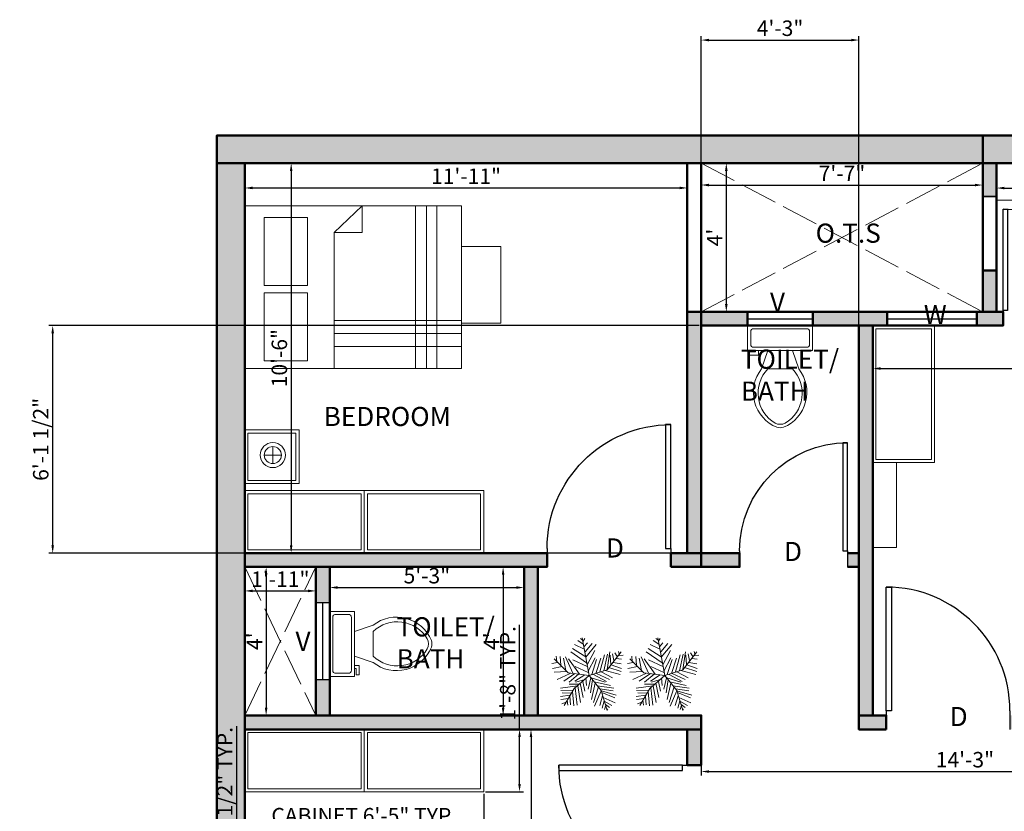
# Model space of a CAD drawing. Units: inches. Extents: x 2227 to 2709, y 1385 to 2029.
# Tile 3 of 4: x 2227 to 2545, y 1773 to 2029. Entities that reach past the tile are written whole.
import ezdxf

# ---------------------------------------------------------------- set-up
doc = ezdxf.new("R2010")
doc.units = ezdxf.units.IN
doc.linetypes.add('ACAD_ISO02W100', pattern=[15, 12, -3])
for name, color, linetype, lineweight in [('A-ANNO-DIMS', 1, 'Continuous', 18), ('A-ANNO-TEXT', 30, 'Continuous', 18), ('A-AREA-IDEN', 30, 'Continuous', 25), ('A-FLOR-FIXT', 9, 'Continuous', 18), ('A-FLOR-OPEN', 8, 'ACAD_ISO02W100', 18), ('A-FURN', 50, 'Continuous', 18), ('A-WALL-HIDN', 160, 'ACAD_ISO02W100', 18), ('A-WALL-PATT', 252, 'Continuous', 13), ('BED', 50, 'Continuous', 18), ('DOOR', 130, 'Continuous', 25), ('TREE', 80, 'Continuous', 13), ('WALL', 160, 'Continuous', 50), ('WIND', 40, 'Continuous', 25)]:
    doc.layers.add(name, color=color, linetype=linetype, lineweight=lineweight)
doc.styles.get("Standard").update_dxf_attribs({"font": 'arial.ttf'})
doc.dimstyles.new('ISO-25', dxfattribs={"dimtxt": 5, "dimasz": 2.5, "dimexe": 1.25, "dimexo": 0.625, "dimtad": 1, "dimdec": 0, "dimlunit": 4, "dimtxsty": 'Standard', "dimcen": 2.5, "dimadec": 0, "dimazin": 0, "dimtfac": 1, "dimtdec": 0, "dimtmove": 0, "dimatfit": 3, "dimfxl": 1, "dimarcsym": 0})

# ---------------------------------------------------------------- blocks, each defined once
blk = doc.blocks.new('*U2')
for p, q in [((0, 0), (0, -6)), ((40, 0), (40, -6))]:
    blk.add_line(p, q)
blk.add_lwpolyline([(0, 0), (0, 40), (1.75, 40), (1.75, 0)], close=True)
blk.add_arc((0, 0), 40, 0, 90)
blk = doc.blocks.new('*U4')
for p, q in [((9.5, -6), (9.5, -2)), ((-10, -8.5), (-8, -8.5)), ((-10, -9.5), (-10, -8.5)), ((-7, -9.5), (-10, -9.5)), ((-8, -8.5), (-8, -8)), ((-7, -8), (-7, -9.5)), ((-4, -8), (-6, -14)), ((4, -8), (6, -14)), ((4, -14), (-4, -14))]:
    blk.add_line(p, q)
blk.add_lwpolyline([(10.5, -8), (10.5, 0), (-10.5, 0), (-10.5, -8)], close=True)
for points in [[(-9.5, -2), (-9.5, -6)], [(8.5, -1), (-8.5, -1)], [(-8.5, -7), (8.5, -7)]]:
    blk.add_lwpolyline(points)
for centre, radius, start, end in [((-8.62, -1.88), 0.884, 81.8699, 188.1301), ((8.62, -1.88), 0.884, 351.8699, 98.1301), ((-8.62, -6.12), 0.884, 171.8699, 278.1301), ((8.62, -6.12), 0.884, 261.8699, 8.1301), ((3.52, -21.58), 12.17, 141.4691, 247.9714), ((4.2, -21.82), 11.33, 136.3677, 238.9468), ((-3.52, -21.58), 12.17, 292.0284, 38.5307), ((-4.2, -21.82), 11.33, 301.053, 43.6321), ((0, -27.88), 4, 245.7318, 294.2682), ((0, -29), 4, 254.8605, 285.1395)]:
    blk.add_arc(centre, radius, start, end)
blk = doc.blocks.new('*U6')
for p, q in [((-7.288, 39.707), (-21.778, 46.673)), ((-8.737, 47.138), (-17.069, 52.711)), ((-10.186, 53.64), (-13.084, 55.962)), ((0, 0), (-10.5, 57)), ((-9.099, 51.782), (-6.563, 55.962)), ((-7.65, 43.423), (-2.578, 49.46)), ((-5.839, 35.992), (4.667, 48.067)), ((-5.114, 27.632), (10.463, 46.673)), ((-3.665, 19.273), (-27.574, 35.527)), ((-5.114, 28.097), (-24.676, 40.636)), ((-2.941, 16.486), (8.652, 37.85)), ((16.259, 5.805), (23.142, 31.348)), ((22.055, 7.198), (27.489, 32.277)), ((27, 9), (48, 36)), ((27.127, 9.056), (31.112, 35.992)), ((31.836, 30.883), (32.561, 16.486)), ((35.096, 32.741), (37.27, 22.524)), ((38.719, 34.134), (41.979, 28.561)), ((43.791, 29.954), (51.036, 30.883)), ((44.153, 36.456), (45.239, 32.741)), ((-47.498, 19.737), (-55.83, 18.344)), ((-31.5, 4.5), (-52.5, 25.5)), ((-48.585, 21.131), (-49.309, 29.026)), ((-43.513, 28.561), (-42.427, 15.558)), ((-38.442, 26.239), (-34.819, 7.663)), ((-35.544, 28.097), (-24.314, 3.947)), ((-14.533, 2.09), (-30.834, 25.31)), ((-24.314, 23.917), (-2.941, 13.7)), ((-1.129, 6.734), (9.014, 26.704)), ((3.942, 1.625), (11.187, 24.381)), ((10.101, 3.483), (17.708, 26.239)), ((33.285, 16.486), (48.862, 10.913)), ((36.183, 19.737), (48.137, 17.88)), ((40.53, 25.775), (48.862, 24.846)), ((-40.615, 13.7), (-55.105, 10.913)), ((-33.37, 6.269), (-52.207, 5.34)), ((-28.299, 3.483), (-47.86, -5.805)), ((-21.416, 3.018), (-38.079, -8.128)), ((0, 0), (-31.5, 4.5)), ((-15.982, 2.09), (-30.11, -9.521)), ((0, 0), (-22.5, -19.5)), ((-6.563, 1.161), (-21.416, -8.128)), ((-20.691, 13.7), (-1.129, 4.876)), ((0, 0), (27, 9)), ((0, 0), (18, -22.5)), ((6.478, 1.625), (26.04, -8.592)), ((11.187, 3.483), (30.749, -5.805)), ((18.07, 5.805), (35.096, -3.483)), ((24.229, 7.663), (46.688, 1.625)), ((29.662, 12.307), (48.137, 6.269)), ((-15.257, -12.772), (-30.11, -12.772)), ((-6.563, -5.805), (-19.967, -9.985)), ((-13.446, -11.378), (-8.737, -32.741)), ((-9.461, -8.592), (-6.201, -23.453)), ((-4.752, -3.483), (-3.665, -14.629)), ((2.493, -3.019), (-1.491, -20.202)), ((1.769, -2.555), (24.229, -9.521)), ((5.029, -6.27), (2.131, -25.775)), ((9.014, -11.378), (3.58, -35.992)), ((7.565, -9.056), (32.198, -14.629)), ((-17.431, -15.094), (-42.789, -18.809)), ((-28.299, -29.026), (-42.789, -31.348)), ((-24.314, -21.596), (-42.427, -22.06)), ((-26.849, -26.24), (-40.253, -25.775)), ((-22.5, -19.5), (-37.5, -45)), ((-25.038, -23.918), (-22.865, -45.281)), ((-20.691, -18.345), (-17.793, -44.352)), ((-17.069, -15.094), (-12.721, -40.172)), ((14.085, -16.951), (6.478, -40.172)), ((18.07, -22.524), (8.289, -45.745)), ((12.274, -15.094), (36.907, -18.809)), ((16.259, -19.738), (36.183, -22.989)), ((18, -22.5), (27, -52.5)), ((18.433, -22.524), (40.53, -29.026)), ((19.157, -25.311), (38.719, -33.206)), ((-30.834, -34.135), (-42.427, -35.528)), ((-34.457, -39.708), (-40.978, -42.494)), ((-32.646, -36.921), (-31.921, -44.352)), ((-29.023, -30.884), (-27.936, -43.887)), ((20.244, -30.419), (15.897, -44.816)), ((22.78, -37.85), (19.519, -48.532)), ((21.331, -32.741), (39.081, -40.636)), ((22.78, -38.314), (34.372, -44.816)), ((24.591, -43.423), (30.749, -47.603)), ((24.591, -45.745), (23.142, -50.854)), ((26.764, -49.925), (28.213, -50.854))]:
    blk.add_line(p, q)
blk = doc.blocks.new('*D9')
at = {"layer": 'A-ANNO-DIMS', "color": 0, "lineweight": -2, "transparency": 16777216}
for p, q in [((2299.71, 1981.71), (2299.71, 1973.09)), ((2442.71, 1981.71), (2442.71, 1973.09)), ((2302.21, 1974.34), (2440.21, 1974.34))]:
    blk.add_line(p, q, dxfattribs=at)
at = {"layer": 'A-ANNO-DIMS', "color": 0, "lineweight": 100, "transparency": 16777216}
for points in [[(2302.21, 1974.76), (2302.21, 1973.93), (2299.71, 1974.34)], [(2440.21, 1974.76), (2440.21, 1973.93), (2442.71, 1974.34)]]:
    blk.add_solid(points, dxfattribs=at)
at = {"layer": 'Defpoints', "color": 0, "lineweight": 100, "transparency": 16777216}
for p in [(2299.71, 1982.33), (2442.71, 1982.33), (2442.71, 1974.34)]:
    blk.add_point(p, dxfattribs=at)
at = {"layer": 'A-ANNO-DIMS', "color": 0, "transparency": 16777216, "insert": (2371.21, 1977.48), "char_height": 5, "attachment_point": 5}
blk.add_mtext('11\'-11"', dxfattribs=at)
blk = doc.blocks.new('*D10')
at = {"layer": 'A-ANNO-DIMS', "color": 0, "lineweight": -2, "transparency": 16777216}
for p, q in [((2300.34, 1982.33), (2315.95, 1982.33)), ((2314.7, 1979.83), (2314.7, 1858.83)), ((2300.34, 1856.33), (2315.95, 1856.33))]:
    blk.add_line(p, q, dxfattribs=at)
at = {"layer": 'A-ANNO-DIMS', "color": 0, "lineweight": 100, "transparency": 16777216}
for points in [[(2314.28, 1979.83), (2315.11, 1979.83), (2314.7, 1982.33)], [(2314.28, 1858.83), (2315.11, 1858.83), (2314.7, 1856.33)]]:
    blk.add_solid(points, dxfattribs=at)
at = {"layer": 'Defpoints', "color": 0, "lineweight": 100, "transparency": 16777216}
for p in [(2299.71, 1982.33), (2299.71, 1856.33), (2314.7, 1856.33)]:
    blk.add_point(p, dxfattribs=at)
at = {"layer": 'A-ANNO-DIMS', "color": 0, "transparency": 16777216, "insert": (2311.52, 1919.33), "char_height": 5, "attachment_point": 5, "rotation": 90}
blk.add_mtext('10\'-6"', dxfattribs=at)
blk = doc.blocks.new('*D11')
at = {"layer": 'A-ANNO-DIMS', "color": 0, "lineweight": -2, "transparency": 16777216}
for p, q in [((2447.21, 1981.71), (2447.21, 1974.03)), ((2538.21, 1981.71), (2538.21, 1974.03)), ((2449.71, 1975.28), (2535.71, 1975.28))]:
    blk.add_line(p, q, dxfattribs=at)
at = {"layer": 'A-ANNO-DIMS', "color": 0, "lineweight": 100, "transparency": 16777216}
for points in [[(2449.71, 1975.7), (2449.71, 1974.86), (2447.21, 1975.28)], [(2535.71, 1975.7), (2535.71, 1974.86), (2538.21, 1975.28)]]:
    blk.add_solid(points, dxfattribs=at)
at = {"layer": 'Defpoints', "color": 0, "lineweight": 100, "transparency": 16777216}
for p in [(2447.21, 1982.33), (2538.21, 1982.33), (2538.21, 1975.28)]:
    blk.add_point(p, dxfattribs=at)
at = {"layer": 'A-ANNO-DIMS', "color": 0, "transparency": 16777216, "insert": (2492.71, 1978.4), "char_height": 5, "attachment_point": 5}
blk.add_mtext('7\'-7"', dxfattribs=at)
blk = doc.blocks.new('*D12')
at = {"layer": 'A-ANNO-DIMS', "color": 0, "lineweight": -2, "transparency": 16777216}
for p, q in [((2447.84, 1982.33), (2456.58, 1982.33)), ((2455.33, 1979.83), (2455.33, 1936.83)), ((2447.84, 1934.33), (2456.58, 1934.33))]:
    blk.add_line(p, q, dxfattribs=at)
at = {"layer": 'A-ANNO-DIMS', "color": 0, "lineweight": 100, "transparency": 16777216}
for points in [[(2454.91, 1979.83), (2455.75, 1979.83), (2455.33, 1982.33)], [(2454.91, 1936.83), (2455.75, 1936.83), (2455.33, 1934.33)]]:
    blk.add_solid(points, dxfattribs=at)
at = {"layer": 'Defpoints', "color": 0, "lineweight": 100, "transparency": 16777216}
for p in [(2447.21, 1982.33), (2447.21, 1934.33), (2455.33, 1934.33)]:
    blk.add_point(p, dxfattribs=at)
at = {"layer": 'A-ANNO-DIMS', "color": 0, "transparency": 16777216, "insert": (2452.21, 1958.33), "char_height": 5, "attachment_point": 5, "rotation": 90}
blk.add_mtext("4'", dxfattribs=at)
blk = doc.blocks.new('*D13')
at = {"layer": 'A-ANNO-DIMS', "color": 0, "lineweight": -2, "transparency": 16777216}
for p, q in [((2542.71, 1981.71), (2542.71, 1973.06)), ((2617.71, 1981.71), (2617.71, 1973.06)), ((2545.21, 1974.31), (2615.21, 1974.31))]:
    blk.add_line(p, q, dxfattribs=at)
at = {"layer": 'A-ANNO-DIMS', "color": 0, "lineweight": 100, "transparency": 16777216}
for points in [[(2545.21, 1974.72), (2545.21, 1973.89), (2542.71, 1974.31)], [(2615.21, 1974.72), (2615.21, 1973.89), (2617.71, 1974.31)]]:
    blk.add_solid(points, dxfattribs=at)
at = {"layer": 'Defpoints', "color": 0, "lineweight": 100, "transparency": 16777216}
for p in [(2542.71, 1982.33), (2617.71, 1982.33), (2617.71, 1974.31)]:
    blk.add_point(p, dxfattribs=at)
at = {"layer": 'A-ANNO-DIMS', "color": 0, "transparency": 16777216, "insert": (2580.21, 1977.49), "char_height": 5, "attachment_point": 5}
blk.add_mtext('6\'-3"', dxfattribs=at)
blk = doc.blocks.new('*D16')
at = {"layer": 'A-ANNO-DIMS', "color": 0, "lineweight": -2, "transparency": 16777216}
for p, q in [((2502.71, 1804.46), (2502.71, 1917.22)), ((2505.21, 1915.97), (2615.21, 1915.97)), ((2617.71, 1804.46), (2617.71, 1917.22))]:
    blk.add_line(p, q, dxfattribs=at)
at = {"layer": 'A-ANNO-DIMS', "color": 0, "lineweight": 100, "transparency": 16777216}
for points in [[(2505.21, 1916.39), (2505.21, 1915.56), (2502.71, 1915.97)], [(2615.21, 1916.39), (2615.21, 1915.56), (2617.71, 1915.97)]]:
    blk.add_solid(points, dxfattribs=at)
at = {"layer": 'Defpoints', "color": 0, "lineweight": 100, "transparency": 16777216}
for p in [(2617.71, 1915.97), (2502.71, 1803.83), (2617.71, 1803.83)]:
    blk.add_point(p, dxfattribs=at)
at = {"layer": 'A-ANNO-DIMS', "color": 0, "transparency": 16777216, "insert": (2560.21, 1919.15), "char_height": 5, "attachment_point": 5}
blk.add_mtext('9\'-7"', dxfattribs=at)
blk = doc.blocks.new('*D17')
at = {"layer": 'A-ANNO-DIMS', "color": 0, "lineweight": -2, "transparency": 16777216}
for p, q in [((2299.71, 1851.21), (2299.71, 1842.84)), ((2322.67, 1851.21), (2322.67, 1842.84)), ((2302.21, 1844.09), (2320.17, 1844.09))]:
    blk.add_line(p, q, dxfattribs=at)
at = {"layer": 'A-ANNO-DIMS', "color": 0, "lineweight": 100, "transparency": 16777216}
for points in [[(2302.21, 1844.51), (2302.21, 1843.68), (2299.71, 1844.09)], [(2320.17, 1844.51), (2320.17, 1843.68), (2322.67, 1844.09)]]:
    blk.add_solid(points, dxfattribs=at)
at = {"layer": 'Defpoints', "color": 0, "lineweight": 100, "transparency": 16777216}
for p in [(2299.71, 1851.83), (2322.67, 1851.83), (2322.67, 1844.09)]:
    blk.add_point(p, dxfattribs=at)
at = {"layer": 'A-ANNO-DIMS', "color": 0, "transparency": 16777216, "insert": (2311.19, 1847.23), "char_height": 5, "attachment_point": 5}
blk.add_mtext('1\'-11"', dxfattribs=at)
blk = doc.blocks.new('*D18')
at = {"layer": 'A-ANNO-DIMS', "color": 0, "lineweight": -2, "transparency": 16777216}
for p, q in [((2300.34, 1851.83), (2307.86, 1851.83)), ((2306.61, 1849.33), (2306.61, 1806.33)), ((2300.34, 1803.83), (2307.86, 1803.83))]:
    blk.add_line(p, q, dxfattribs=at)
at = {"layer": 'A-ANNO-DIMS', "color": 0, "lineweight": 100, "transparency": 16777216}
for points in [[(2306.19, 1849.33), (2307.02, 1849.33), (2306.61, 1851.83)], [(2306.19, 1806.33), (2307.02, 1806.33), (2306.61, 1803.83)]]:
    blk.add_solid(points, dxfattribs=at)
at = {"layer": 'Defpoints', "color": 0, "lineweight": 100, "transparency": 16777216}
for p in [(2299.71, 1851.83), (2299.71, 1803.83), (2306.61, 1803.83)]:
    blk.add_point(p, dxfattribs=at)
at = {"layer": 'A-ANNO-DIMS', "color": 0, "transparency": 16777216, "insert": (2303.48, 1827.83), "char_height": 5, "attachment_point": 5, "rotation": 90}
blk.add_mtext("4'", dxfattribs=at)
blk = doc.blocks.new('*D19')
at = {"layer": 'A-ANNO-DIMS', "color": 0, "lineweight": -2, "transparency": 16777216}
for p, q in [((2327.17, 1851.21), (2327.17, 1843.93)), ((2389.95, 1851.21), (2389.95, 1843.93)), ((2329.67, 1845.18), (2387.45, 1845.18))]:
    blk.add_line(p, q, dxfattribs=at)
at = {"layer": 'A-ANNO-DIMS', "color": 0, "lineweight": 100, "transparency": 16777216}
for points in [[(2329.67, 1845.6), (2329.67, 1844.77), (2327.17, 1845.18)], [(2387.45, 1845.6), (2387.45, 1844.77), (2389.95, 1845.18)]]:
    blk.add_solid(points, dxfattribs=at)
at = {"layer": 'Defpoints', "color": 0, "lineweight": 100, "transparency": 16777216}
for p in [(2327.17, 1851.83), (2389.95, 1851.83), (2389.95, 1845.18)]:
    blk.add_point(p, dxfattribs=at)
at = {"layer": 'A-ANNO-DIMS', "color": 0, "transparency": 16777216, "insert": (2358.56, 1848.36), "char_height": 5, "attachment_point": 5}
blk.add_mtext('5\'-3"', dxfattribs=at)
blk = doc.blocks.new('*D20')
at = {"layer": 'A-ANNO-DIMS', "color": 0, "lineweight": -2, "transparency": 16777216}
for p, q in [((2388.09, 1851.83), (2381.95, 1851.83)), ((2383.2, 1849.33), (2383.2, 1806.33)), ((2388.09, 1803.83), (2381.95, 1803.83))]:
    blk.add_line(p, q, dxfattribs=at)
at = {"layer": 'A-ANNO-DIMS', "color": 0, "lineweight": 100, "transparency": 16777216}
for points in [[(2382.79, 1849.33), (2383.62, 1849.33), (2383.2, 1851.83)], [(2382.79, 1806.33), (2383.62, 1806.33), (2383.2, 1803.83)]]:
    blk.add_solid(points, dxfattribs=at)
at = {"layer": 'Defpoints', "color": 0, "lineweight": 100, "transparency": 16777216}
for p in [(2388.72, 1851.83), (2383.2, 1803.83), (2388.72, 1803.83)]:
    blk.add_point(p, dxfattribs=at)
at = {"layer": 'A-ANNO-DIMS', "color": 0, "transparency": 16777216, "insert": (2380.08, 1827.83), "char_height": 5, "attachment_point": 5, "rotation": 90}
blk.add_mtext("4'", dxfattribs=at)
blk = doc.blocks.new('*D21')
at = {"layer": 'A-ANNO-DIMS', "color": 0, "lineweight": -2, "transparency": 16777216}
for p, q in [((2300.34, 1799.33), (2393.46, 1799.33)), ((2392.21, 1796.83), (2392.21, 1669.83)), ((2300.34, 1667.33), (2393.46, 1667.33))]:
    blk.add_line(p, q, dxfattribs=at)
at = {"layer": 'A-ANNO-DIMS', "color": 0, "lineweight": 100, "transparency": 16777216}
for points in [[(2391.79, 1796.83), (2392.62, 1796.83), (2392.21, 1799.33)], [(2391.79, 1669.83), (2392.62, 1669.83), (2392.21, 1667.33)]]:
    blk.add_solid(points, dxfattribs=at)
at = {"layer": 'Defpoints', "color": 0, "lineweight": 100, "transparency": 16777216}
for p in [(2299.71, 1799.33), (2299.71, 1667.33), (2392.21, 1667.33)]:
    blk.add_point(p, dxfattribs=at)
at = {"layer": 'A-ANNO-DIMS', "color": 0, "transparency": 16777216, "insert": (2389.07, 1733.33), "char_height": 5, "attachment_point": 5, "rotation": 90}
blk.add_mtext("11'", dxfattribs=at)
blk = doc.blocks.new('*D29')
at = {"layer": 'A-ANNO-DIMS', "color": 0, "lineweight": -2, "transparency": 16777216}
for p, q in [((2447.21, 1798.71), (2447.21, 1784.46)), ((2617.71, 1798.71), (2617.71, 1784.46)), ((2449.71, 1785.71), (2615.21, 1785.71))]:
    blk.add_line(p, q, dxfattribs=at)
at = {"layer": 'A-ANNO-DIMS', "color": 0, "lineweight": 100, "transparency": 16777216}
for points in [[(2449.71, 1786.12), (2449.71, 1785.29), (2447.21, 1785.71)], [(2615.21, 1786.12), (2615.21, 1785.29), (2617.71, 1785.71)]]:
    blk.add_solid(points, dxfattribs=at)
at = {"layer": 'Defpoints', "color": 0, "lineweight": 100, "transparency": 16777216}
for p in [(2447.21, 1799.33), (2617.71, 1799.33), (2617.71, 1785.71)]:
    blk.add_point(p, dxfattribs=at)
at = {"layer": 'A-ANNO-DIMS', "color": 0, "transparency": 16777216, "insert": (2532.46, 1788.89), "char_height": 5, "attachment_point": 5}
blk.add_mtext('14\'-3"', dxfattribs=at)
blk = doc.blocks.new('BED-DOUBLE')
for p, q in [((37.96, 0), (28.86, -8.71)), ((37.96, -8.71), (37.96, 0)), ((55.17, -52.67), (55.17, 0)), ((58.68, -52.67), (58.68, 0)), ((62.04, -52.67), (62.04, 0)), ((28.86, -52.67), (28.86, -8.71)), ((28.86, -8.71), (37.96, -8.71)), ((28.86, -37.1), (70.02, -37.1)), ((28.86, -41.31), (70.02, -41.31)), ((28.86, -45.51), (70.02, -45.51))]:
    blk.add_line(p, q)
for points in [[(0, 0), (70.02, 0), (70.02, -52.67), (0, -52.67)], [(6.26, -25.79), (20.3, -25.79), (20.3, -3.78), (6.26, -3.78)], [(70.02, -38), (82.72, -38), (82.72, -13.23), (70.02, -13.23)], [(6.26, -50.18), (20.3, -50.18), (20.3, -28.17), (6.26, -28.17)]]:
    blk.add_lwpolyline(points, close=True)
blk = doc.blocks.new('CABINET-DOUBLE')
blk.add_line((38.61, 20.17), (38.61, 0))
for points in [[(0, 0), (77.21, 0), (77.21, 20.17), (0, 20.17)], [(0, 20.17), (38.61, 20.17), (38.61, 0), (0, 0)], [(1, 19.17), (37.61, 19.17), (37.61, 1), (1, 1)], [(77.21, 20.17), (38.61, 20.17), (38.61, 0), (77.21, 0)], [(76.21, 19.17), (39.61, 19.17), (39.61, 1), (76.21, 1)]]:
    blk.add_lwpolyline(points, close=True)
blk = doc.blocks.new('NIGHTSTAND')
for p, q in [((9.06, 6.42), (9.06, 11.97)), ((6.28, 9.2), (11.83, 9.2))]:
    blk.add_line(p, q)
for points in [[(0, 0), (17.54, 0), (17.54, 17.32), (0, 17.32)], [(1, 1), (16.54, 1), (16.54, 16.32), (1, 16.32)]]:
    blk.add_lwpolyline(points, close=True)
for radius in [4.05, 2.77]:
    blk.add_circle((9.06, 9.2), radius)
blk = doc.blocks.new('*D39')
at = {"layer": 'A-ANNO-DIMS', "color": 0, "lineweight": -2, "transparency": 16777216}
for p, q in [((2299.71, 1778.54), (2299.71, 1766.33)), ((2376.93, 1778.54), (2376.93, 1766.33)), ((2302.21, 1767.58), (2374.43, 1767.58))]:
    blk.add_line(p, q, dxfattribs=at)
at = {"layer": 'A-ANNO-DIMS', "color": 0, "lineweight": 100, "transparency": 16777216}
for points in [[(2302.21, 1768), (2302.21, 1767.16), (2299.71, 1767.58)], [(2374.43, 1768), (2374.43, 1767.16), (2376.93, 1767.58)]]:
    blk.add_solid(points, dxfattribs=at)
at = {"layer": 'Defpoints', "color": 0, "lineweight": 100, "transparency": 16777216}
for p in [(2299.71, 1779.16), (2376.93, 1779.16), (2376.93, 1767.58)]:
    blk.add_point(p, dxfattribs=at)
at = {"layer": 'A-ANNO-DIMS', "color": 0, "transparency": 16777216, "insert": (2338.32, 1770.79), "char_height": 5, "attachment_point": 5}
blk.add_mtext('CABINET 6\'-5" TYP.', dxfattribs=at)
blk = doc.blocks.new('*D40')
at = {"layer": 'A-ANNO-DIMS', "color": 0, "lineweight": -2, "transparency": 16777216}
for p, q in [((2388.51, 1799.33), (2388.51, 1833.09)), ((2377.55, 1799.33), (2389.76, 1799.33)), ((2388.51, 1781.66), (2388.51, 1796.83)), ((2377.55, 1779.16), (2389.76, 1779.16))]:
    blk.add_line(p, q, dxfattribs=at)
at = {"layer": 'A-ANNO-DIMS', "color": 0, "lineweight": 100, "transparency": 16777216}
for points in [[(2388.09, 1796.83), (2388.92, 1796.83), (2388.51, 1799.33)], [(2388.09, 1781.66), (2388.92, 1781.66), (2388.51, 1779.16)]]:
    blk.add_solid(points, dxfattribs=at)
at = {"layer": 'Defpoints', "color": 0, "lineweight": 100, "transparency": 16777216}
for p in [(2376.93, 1799.33), (2388.51, 1799.33), (2376.93, 1779.16)]:
    blk.add_point(p, dxfattribs=at)
at = {"layer": 'A-ANNO-DIMS', "color": 0, "transparency": 16777216, "insert": (2385.33, 1817.46), "char_height": 5, "attachment_point": 5, "rotation": 90}
blk.add_mtext('1\'-8" TYP.', dxfattribs=at)
blk = doc.blocks.new('*D41')
at = {"layer": 'A-ANNO-DIMS', "color": 0, "lineweight": -2, "transparency": 16777216}
for p, q in [((2299.71, 1755.65), (2299.71, 1758.91)), ((2302.21, 1757.66), (2314.75, 1757.66)), ((2317.25, 1755.65), (2317.25, 1758.91)), ((2317.25, 1757.66), (2410.23, 1757.66))]:
    blk.add_line(p, q, dxfattribs=at)
at = {"layer": 'A-ANNO-DIMS', "color": 0, "lineweight": 100, "transparency": 16777216}
for points in [[(2302.21, 1758.07), (2302.21, 1757.24), (2299.71, 1757.66)], [(2314.75, 1758.07), (2314.75, 1757.24), (2317.25, 1757.66)]]:
    blk.add_solid(points, dxfattribs=at)
at = {"layer": 'Defpoints', "color": 0, "lineweight": 100, "transparency": 16777216}
for p in [(2317.25, 1757.66), (2299.71, 1755.03), (2317.25, 1755.03)]:
    blk.add_point(p, dxfattribs=at)
at = {"layer": 'A-ANNO-DIMS', "color": 0, "transparency": 16777216, "insert": (2364.99, 1760.87), "char_height": 5, "attachment_point": 5}
blk.add_mtext('NIGHTSTAND 1\'-5 1/2" TYP.', dxfattribs=at)
blk = doc.blocks.new('*D42')
at = {"layer": 'A-ANNO-DIMS', "color": 0, "lineweight": -2, "transparency": 16777216}
for p, q in [((2297.08, 1755.03), (2297.08, 1800.43)), ((2299.09, 1755.03), (2295.83, 1755.03)), ((2297.08, 1740.21), (2297.08, 1752.53)), ((2299.09, 1737.71), (2295.83, 1737.71))]:
    blk.add_line(p, q, dxfattribs=at)
at = {"layer": 'A-ANNO-DIMS', "color": 0, "lineweight": 100, "transparency": 16777216}
for points in [[(2296.67, 1752.53), (2297.5, 1752.53), (2297.08, 1755.03)], [(2296.67, 1740.21), (2297.5, 1740.21), (2297.08, 1737.71)]]:
    blk.add_solid(points, dxfattribs=at)
at = {"layer": 'Defpoints', "color": 0, "lineweight": 100, "transparency": 16777216}
for p in [(2297.08, 1755.03), (2299.71, 1755.03), (2299.71, 1737.71)]:
    blk.add_point(p, dxfattribs=at)
at = {"layer": 'A-ANNO-DIMS', "color": 0, "transparency": 16777216, "insert": (2293.87, 1778.98), "char_height": 5, "attachment_point": 5, "rotation": 90}
blk.add_mtext('1\'-5 1/2" TYP.', dxfattribs=at)
blk = doc.blocks.new('*D49')
at = {"layer": 'A-ANNO-DIMS', "color": 0, "lineweight": -2, "transparency": 16777216}
for p, q in [((2447.21, 1856.96), (2447.21, 2023.39)), ((2449.71, 2022.14), (2495.71, 2022.14)), ((2498.21, 1856.96), (2498.21, 2023.39))]:
    blk.add_line(p, q, dxfattribs=at)
at = {"layer": 'A-ANNO-DIMS', "color": 0, "lineweight": 100, "transparency": 16777216}
for points in [[(2449.71, 2022.56), (2449.71, 2021.72), (2447.21, 2022.14)], [(2495.71, 2022.56), (2495.71, 2021.72), (2498.21, 2022.14)]]:
    blk.add_solid(points, dxfattribs=at)
at = {"layer": 'Defpoints', "color": 0, "lineweight": 100, "transparency": 16777216}
for p in [(2498.21, 2022.14), (2447.21, 1856.33), (2498.21, 1856.33)]:
    blk.add_point(p, dxfattribs=at)
at = {"layer": 'A-ANNO-DIMS', "color": 0, "transparency": 16777216, "insert": (2472.71, 2025.32), "char_height": 5, "attachment_point": 5}
blk.add_mtext('4\'-3"', dxfattribs=at)
blk = doc.blocks.new('*D50')
at = {"layer": 'A-ANNO-DIMS', "color": 0, "lineweight": -2, "transparency": 16777216}
for p, q in [((2446.59, 1929.83), (2236.37, 1929.83)), ((2237.62, 1858.83), (2237.62, 1927.33)), ((2446.59, 1856.33), (2236.37, 1856.33))]:
    blk.add_line(p, q, dxfattribs=at)
at = {"layer": 'A-ANNO-DIMS', "color": 0, "lineweight": 100, "transparency": 16777216}
for points in [[(2237.2, 1927.33), (2238.04, 1927.33), (2237.62, 1929.83)], [(2237.2, 1858.83), (2238.04, 1858.83), (2237.62, 1856.33)]]:
    blk.add_solid(points, dxfattribs=at)
at = {"layer": 'Defpoints', "color": 0, "lineweight": 100, "transparency": 16777216}
for p in [(2237.62, 1929.83), (2447.21, 1929.83), (2447.21, 1856.33)]:
    blk.add_point(p, dxfattribs=at)
at = {"layer": 'A-ANNO-DIMS', "color": 0, "transparency": 16777216, "insert": (2234.41, 1893.08), "char_height": 5, "attachment_point": 5, "rotation": 90}
blk.add_mtext('6\'-1 1/2"', dxfattribs=at)

msp = doc.modelspace()

# ---------------------------------------------------------------- hatches: boundary and pattern name
at = {"layer": 'A-WALL-PATT'}
h = msp.add_hatch(color=256, dxfattribs=at)
h.dxf.hatch_style = 1
h.paths.add_polyline_path([(2538.21, 1991.33), (2290.71, 1991.33), (2290.71, 1982.33), (2299.71, 1982.33), (2538.21, 1982.33)])
h.paths.add_polyline_path([(2299.71, 1982.33), (2290.71, 1982.33), (2290.71, 1424.33), (2299.71, 1424.33)])
h.paths.add_polyline_path([(2347.13, 1424.33), (2290.71, 1424.33), (2290.71, 1415.33), (2347.13, 1415.33)])
h.paths.add_polyline_path([(2447.21, 1424.33), (2402.93, 1424.33), (2402.93, 1415.33), (2447.21, 1415.33)])
h.paths.add_polyline_path([(2447.21, 1597.83), (2442.71, 1597.83), (2442.71, 1424.33), (2447.21, 1424.33)])
h.paths.add_polyline_path([(2396.41, 1528.83), (2299.71, 1528.83), (2299.71, 1524.33), (2396.41, 1524.33)])
h.paths.add_polyline_path([(2442.71, 1528.83), (2436.41, 1528.83), (2436.41, 1524.33), (2442.71, 1524.33)])
h.paths.add_polyline_path([(2345.64, 1667.33), (2299.71, 1667.33), (2299.71, 1662.83), (2345.64, 1662.83)])
h.paths.add_polyline_path([(2447.21, 1747.77), (2442.71, 1747.77), (2442.71, 1662.83), (2447.21, 1662.83)])
h.paths.add_polyline_path([(2442.71, 1667.33), (2401.29, 1667.33), (2401.29, 1662.83), (2442.71, 1662.83)])
h.paths.add_polyline_path([(2447.21, 1803.83), (2299.71, 1803.83), (2299.71, 1799.33), (2447.21, 1799.33)])
h.paths.add_polyline_path([(2447.21, 1799.33), (2442.71, 1799.33), (2442.71, 1787.77), (2447.21, 1787.77)])
h.paths.add_polyline_path([(2394.45, 1851.83), (2389.95, 1851.83), (2389.95, 1803.83), (2394.45, 1803.83)])
h.paths.add_polyline_path([(2327.17, 1851.83), (2322.67, 1851.83), (2322.67, 1840.2), (2327.17, 1840.2)])
h.paths.add_polyline_path([(2327.17, 1815.42), (2322.67, 1815.42), (2322.67, 1803.83), (2327.17, 1803.83)])
h.paths.add_polyline_path([(2397.41, 1856.33), (2299.71, 1856.33), (2299.71, 1851.83), (2397.41, 1851.83)])
h.paths.add_polyline_path([(2447.21, 1856.33), (2437.41, 1856.33), (2437.41, 1851.83), (2447.21, 1851.83)])
h.paths.add_polyline_path([(2447.21, 1934.33), (2442.71, 1934.33), (2442.71, 1856.33), (2447.21, 1856.33)])
h.paths.add_polyline_path([(2459.62, 1856.33), (2447.21, 1856.33), (2447.21, 1851.83), (2459.62, 1851.83)])
h.paths.add_polyline_path([(2498.21, 1856.33), (2494.53, 1856.33), (2494.53, 1851.83), (2498.21, 1851.83)])
h.paths.add_polyline_path([(2462.23, 1934.33), (2447.21, 1934.33), (2447.21, 1929.83), (2462.23, 1929.83)])
h.paths.add_polyline_path([(2507.32, 1934.33), (2483.3, 1934.33), (2483.3, 1929.83), (2507.32, 1929.83)])
h.paths.add_polyline_path([(2542.71, 1947.66), (2538.21, 1947.66), (2538.21, 1934.33), (2542.71, 1934.33)])
h.paths.add_polyline_path([(2544.78, 1934.33), (2536.35, 1934.33), (2536.35, 1929.83), (2544.78, 1929.83)])
h.paths.add_polyline_path([(2542.71, 1982.33), (2538.21, 1982.33), (2538.21, 1971.57), (2542.71, 1971.57)])
h.paths.add_polyline_path([(2346.6, 1815.57), (2382.82, 1815.57), (2382.82, 1838.66), (2346.6, 1838.66)], flags=9)
h.paths.add_polyline_path([(2457.86, 1902.08), (2494.08, 1902.08), (2494.08, 1925.17), (2457.86, 1925.17)], flags=9)
h.paths.add_polyline_path([(2500.39, 1690.49), (2545.31, 1690.49), (2545.31, 1713.58), (2500.39, 1713.58)], flags=9)
h.paths.add_polyline_path([(2528.08, 1476.92), (2562.42, 1476.92), (2562.42, 1489.69), (2528.08, 1489.69)], flags=9)
h.paths.add_polyline_path([(2349.07, 1476.93), (2390.15, 1476.93), (2390.15, 1489.69), (2349.07, 1489.69)], flags=9)
h.paths.add_polyline_path([(2347.99, 1586.39), (2381.37, 1586.39), (2381.37, 1609.48), (2347.99, 1609.48)], flags=9)
h.paths.add_polyline_path([(2328.07, 1742.46), (2375.88, 1742.46), (2375.88, 1755.23), (2328.07, 1755.23)], flags=9)
h.paths.add_polyline_path([(2556.42, 1893.75), (2604.23, 1893.75), (2604.23, 1906.51), (2556.42, 1906.51)], flags=9)
h.paths.add_polyline_path([(2323.02, 1893.88), (2370.83, 1893.88), (2370.83, 1906.64), (2323.02, 1906.64)], flags=9)
h.paths.add_polyline_path([(2562.19, 1958.77), (2598.41, 1958.77), (2598.41, 1981.86), (2562.19, 1981.86)], flags=9)
h.paths.add_polyline_path([(2482.23, 1953.14), (2507.92, 1953.14), (2507.92, 1965.9), (2482.23, 1965.9)], flags=9)
h = msp.add_hatch(color=256, dxfattribs=at)
h.dxf.hatch_style = 1
h.paths.add_polyline_path([(2617.71, 1991.33), (2538.21, 1991.33), (2538.21, 1982.33), (2617.71, 1982.33)])
h.paths.add_polyline_path([(2626.71, 1991.33), (2617.71, 1991.33), (2617.71, 1982.33), (2617.71, 1415.33), (2626.71, 1415.33)])
h.paths.add_polyline_path([(2617.71, 1934.33), (2577.48, 1934.33), (2577.48, 1929.83), (2617.71, 1929.83)])
h.paths.add_polyline_path([(2502.71, 1929.83), (2498.21, 1929.83), (2498.21, 1803.83), (2502.71, 1803.83)])
h.paths.add_polyline_path([(2617.71, 1803.83), (2547.01, 1803.83), (2547.01, 1799.33), (2617.71, 1799.33)])
h.paths.add_polyline_path([(2507.01, 1803.83), (2498.21, 1803.83), (2498.21, 1799.33), (2507.01, 1799.33)])
h.paths.add_polyline_path([(2617.71, 1602.33), (2607.17, 1602.33), (2607.17, 1601.18), (2607.17, 1597.83), (2617.71, 1597.83)])

# ---------------------------------------------------------------- linework, layer by layer
at = {"layer": 'A-FLOR-FIXT'}
msp.add_lwpolyline([(2542.71, 1982.33), (2564.37, 1982.33), (2564.37, 1970.37), (2542.71, 1970.37)], close=True, dxfattribs=at)
at = {"layer": 'A-FLOR-OPEN'}
for p, q in [((2447.21, 1934.33), (2538.21, 1982.33)), ((2447.21, 1982.33), (2538.21, 1934.33)), ((2299.71, 1803.83), (2322.67, 1851.83)), ((2299.71, 1851.83), (2322.67, 1803.83))]:
    msp.add_line(p, q, dxfattribs=at)
at = {"layer": 'A-FURN'}
for points in [[(2502.71, 1929.83), (2522.63, 1929.83), (2522.63, 1885.62), (2502.71, 1885.62)], [(2503.71, 1928.83), (2521.63, 1928.83), (2521.63, 1886.62), (2503.71, 1886.62)], [(2502.71, 1885.62), (2510.33, 1885.62), (2510.33, 1858.15), (2502.71, 1858.15)]]:
    msp.add_lwpolyline(points, close=True, dxfattribs=at)
at = {"layer": 'A-WALL-HIDN'}
msp.add_line((2447.21, 1799.33), (2447.21, 1803.83), dxfattribs=at)
at = {"layer": 'WALL'}
for p, q in [((2290.71, 1991.33), (2626.71, 1991.33)), ((2290.71, 1415.33), (2290.71, 1991.33)), ((2538.21, 1982.33), (2538.21, 1991.33)), ((2299.71, 1982.33), (2442.71, 1982.33)), ((2442.71, 1982.33), (2442.71, 1856.33)), ((2447.21, 1982.33), (2447.21, 1851.83)), ((2447.21, 1982.33), (2538.21, 1982.33)), ((2538.21, 1982.33), (2538.21, 1934.33)), ((2542.71, 1982.33), (2542.71, 1934.33)), ((2538.21, 1934.33), (2447.21, 1934.33)), ((2538.21, 1934.33), (2544.78, 1934.33)), ((2542.71, 1929.83), (2447.21, 1929.83)), ((2498.21, 1799.33), (2498.21, 1929.83)), ((2502.71, 1803.83), (2502.71, 1929.83)), ((2542.71, 1929.83), (2544.78, 1929.83)), ((2397.41, 1856.33), (2299.71, 1856.33)), ((2442.71, 1856.33), (2437.41, 1856.33)), ((2442.71, 1856.33), (2459.62, 1856.33)), ((2494.53, 1856.33), (2498.21, 1856.33)), ((2299.71, 1851.83), (2347.71, 1851.83)), ((2299.71, 1851.83), (2371.71, 1851.83)), ((2397.41, 1851.83), (2299.71, 1851.83)), ((2322.67, 1851.83), (2322.67, 1803.83)), ((2327.17, 1851.83), (2327.17, 1803.83)), ((2389.95, 1851.83), (2389.95, 1803.83)), ((2394.45, 1851.83), (2394.45, 1803.83)), ((2447.21, 1851.83), (2437.41, 1851.83)), ((2447.21, 1851.83), (2459.62, 1851.83)), ((2494.53, 1851.83), (2498.21, 1851.83)), ((2347.71, 1803.83), (2299.71, 1803.83)), ((2299.71, 1803.83), (2371.71, 1803.83)), ((2347.71, 1803.83), (2379.75, 1803.83)), ((2447.21, 1803.83), (2352.21, 1803.83)), ((2502.71, 1803.83), (2498.21, 1803.83)), ((2507.01, 1803.83), (2502.71, 1803.83)), ((2447.21, 1799.33), (2299.71, 1799.33)), ((2299.71, 1799.33), (2442.71, 1799.33)), ((2442.71, 1799.33), (2442.71, 1787.77)), ((2447.21, 1799.33), (2447.21, 1787.77)), ((2507.01, 1799.33), (2498.21, 1799.33))]:
    msp.add_line(p, q, dxfattribs=at)
for points in [[(2447.21, 1415.33), (2290.71, 1415.33), (2290.71, 1991.33), (2626.71, 1991.33), (2626.71, 1415.33), (2617.71, 1415.33)], [(2447.21, 1424.33), (2299.71, 1424.33), (2299.71, 1982.33), (2617.71, 1982.33), (2617.71, 1424.33)]]:
    msp.add_lwpolyline(points, dxfattribs=at)
for points in [[(2538.21, 1982.33), (2290.71, 1982.33), (2290.71, 1991.33), (2538.21, 1991.33)], [(2538.21, 1991.33), (2617.71, 1991.33), (2617.71, 1982.33), (2538.21, 1982.33)], [(2290.71, 1982.33), (2299.71, 1982.33), (2299.71, 1424.33), (2290.71, 1424.33)], [(2538.21, 1947.66), (2542.71, 1947.66), (2542.71, 1934.33), (2538.21, 1934.33)], [(2442.71, 1856.33), (2447.21, 1856.33), (2447.21, 1934.33), (2442.71, 1934.33)], [(2447.21, 1929.83), (2462.23, 1929.83), (2462.23, 1934.33), (2447.21, 1934.33)], [(2483.3, 1934.33), (2507.32, 1934.33), (2507.32, 1929.83), (2483.3, 1929.83)], [(2536.35, 1934.33), (2544.78, 1934.33), (2544.78, 1929.83), (2536.35, 1929.83)], [(2498.21, 1803.83), (2502.71, 1803.83), (2502.71, 1929.83), (2498.21, 1929.83)], [(2299.71, 1851.83), (2397.41, 1851.83), (2397.41, 1856.33), (2299.71, 1856.33)], [(2437.41, 1851.83), (2459.62, 1851.83), (2459.62, 1856.33), (2437.41, 1856.33)], [(2389.95, 1851.83), (2394.45, 1851.83), (2394.45, 1803.83), (2389.95, 1803.83)], [(2299.71, 1799.33), (2447.21, 1799.33), (2447.21, 1803.83), (2299.71, 1803.83)], [(2507.01, 1799.33), (2498.21, 1799.33), (2498.21, 1803.83), (2507.01, 1803.83)], [(2447.21, 1787.77), (2442.71, 1787.77), (2442.71, 1799.33), (2447.21, 1799.33)]]:
    msp.add_lwpolyline(points, close=True, dxfattribs=at)
at = {"layer": 'WIND'}
for p, q in [((2462.23, 1932.08), (2483.3, 1932.08)), ((2507.32, 1932.08), (2536.35, 1932.08)), ((2324.92, 1815.42), (2324.92, 1840.2))]:
    msp.add_line(p, q, dxfattribs=at)
for points in [[(2442.71, 1982.33), (2447.21, 1982.33), (2447.21, 1934.33), (2442.71, 1934.33)], [(2538.21, 1971.57), (2542.71, 1971.57), (2542.71, 1947.66), (2538.21, 1947.66)], [(2538.21, 1947.66), (2542.71, 1947.66), (2542.71, 1971.57), (2538.21, 1971.57)], [(2447.21, 1934.33), (2442.71, 1934.33), (2442.71, 1934.33), (2447.21, 1934.33)], [(2444.96, 1934.33), (2442.71, 1934.33), (2442.71, 1934.33), (2444.96, 1934.33)], [(2462.23, 1929.83), (2483.3, 1929.83), (2483.3, 1934.33), (2462.23, 1934.33)], [(2536.35, 1929.83), (2507.32, 1929.83), (2507.32, 1934.33), (2536.35, 1934.33)], [(2322.67, 1815.42), (2327.17, 1815.42), (2327.17, 1840.2), (2322.67, 1840.2)]]:
    msp.add_lwpolyline(points, close=True, dxfattribs=at)

# ---------------------------------------------------------------- block references
at = {"layer": 'A-FLOR-FIXT'}
msp.add_blockref('*U4', (2472.73, 1929.83), dxfattribs=at)
at = {"layer": 'A-FLOR-FIXT', "rotation": 90.00000000000003}
msp.add_blockref('*U4', (2327.17, 1826.98), dxfattribs=at)
at = {"layer": 'A-FURN'}
for name, p in [('NIGHTSTAND', (2299.71, 1878.8)), ('CABINET-DOUBLE', (2299.71, 1856.33)), ('CABINET-DOUBLE', (2299.71, 1779.16))]:
    msp.add_blockref(name, p, dxfattribs=at)
at = {"layer": 'BED'}
msp.add_blockref('BED-DOUBLE', (2299.71, 1968.61), dxfattribs=at)
at = {"layer": 'DOOR'}
for p, xscale, yscale, zscale in [((2544.78, 1934.74), 0.8174402911474247, 0.8174402911474247, 0.8174402911474247), ((2494.53, 1857.07), -0.8726599657042747, 0.8726599657042747, 0.8726599657042747)]:
    msp.add_blockref('*U2', p, dxfattribs=dict(at, xscale=xscale, yscale=yscale, zscale=zscale))
at = {"layer": 'DOOR', "xscale": -1}
msp.add_blockref('*U2', (2437.41, 1857.83), dxfattribs=at)
at = {"layer": 'DOOR'}
msp.add_blockref('*U2', (2507.01, 1805.33), dxfattribs=at)
at = {"layer": 'DOOR', "xscale": -1, "rotation": 90}
msp.add_blockref('*U2', (2441.21, 1787.77), dxfattribs=at)
at = {"layer": 'TREE', "xscale": 0.2153773147918839, "yscale": 0.2153773147918839, "zscale": 0.2153773147918839}
for p in [(2410.98, 1816.7), (2435.42, 1816.7)]:
    msp.add_blockref('*U6', p, dxfattribs=at)

# ---------------------------------------------------------------- texts
at = {"layer": 'A-ANNO-TEXT', "char_height": 6.19, "attachment_point": 1}
for s, insert in [('V', (2469.45, 1940.53)), ('W', (2519.15, 1936.55)), ('D', (2416.42, 1861.08)), ('D', (2473.99, 1859.94)), ('V', (2316.09, 1830.9)), ('D', (2527.54, 1806.58))]:
    msp.add_mtext_dynamic_manual_height_columns(s, width=156.7329, gutter_width=30.97, heights=[0], dxfattribs=dict(at, insert=insert))
at = {"layer": 'A-AREA-IDEN', "char_height": 6.194, "attachment_point": 1}
for s, insert in [('O.T.S', (2484.2, 1962.83)), ('TOILET/\\PBATH', (2460.04, 1922.09)), ('BEDROOM', (2325.2, 1903.57)), ('TOILET/\\PBATH', (2348.78, 1835.58))]:
    msp.add_mtext_dynamic_manual_height_columns(s, width=156.7329, gutter_width=30.97, heights=[0], dxfattribs=dict(at, insert=insert))

# ---------------------------------------------------------------- dimensions: what is measured, and where the dimension line sits
at = {"layer": 'A-ANNO-DIMS'}
for base, p1, p2, override, picture, middle in [((2498.21, 2022.14), (2447.21, 1856.33), (2498.21, 1856.33), {"dimdec": 1, "dimlfac": 1, "dimrnd": 0, "dimzin": 1, "dimdsep": 46, "dimlunit": 4, "dimfrac": 2}, '*D49', (2472.71, 2025.32)), ((2442.71, 1974.34), (2299.71, 1982.33), (2442.71, 1982.33), {"dimclrd": 0, "dimclre": 0, "dimclrt": 0}, '*D9', (2371.21, 1977.48)), ((2538.21, 1975.28), (2447.21, 1982.33), (2538.21, 1982.33), {"dimclrd": 0, "dimclre": 0, "dimclrt": 0}, '*D11', (2492.71, 1978.4)), ((2617.71, 1974.31), (2542.71, 1982.33), (2617.71, 1982.33), {"dimclrd": 0, "dimclre": 0, "dimclrt": 0}, '*D13', (2580.21, 1977.49)), ((2617.71, 1915.97), (2502.71, 1803.83), (2617.71, 1803.83), {"dimclrd": 0, "dimclre": 0, "dimclrt": 0}, '*D16', (2560.21, 1919.15)), ((2322.67, 1844.09), (2299.71, 1851.83), (2322.67, 1851.83), {"dimclrd": 0, "dimclre": 0, "dimclrt": 0}, '*D17', (2311.19, 1847.23)), ((2389.95, 1845.18), (2327.17, 1851.83), (2389.95, 1851.83), {"dimclrd": 0, "dimclre": 0, "dimclrt": 0}, '*D19', (2358.56, 1848.36)), ((2617.71377381, 1785.70618657), (2447.21377381, 1799.33305883), (2617.71377381, 1799.33305883), {"dimclrd": 0, "dimclre": 0, "dimclrt": 0}, '*D29', (2532.46377381, 1788.88575683))]:
    dim = msp.add_linear_dim(base=base, p1=p1, p2=p2, dimstyle='ISO-25', override=override, dxfattribs=at)
    dim.commit()
    dim.dimension.update_dxf_attribs({"geometry": picture, "text_midpoint": middle})
for base, p1, p2, override, picture, middle in [((2314.7, 1856.33), (2299.71, 1982.33), (2299.71, 1856.33), {"dimclrd": 0, "dimclre": 0, "dimclrt": 0}, '*D10', (2311.52, 1919.33)), ((2455.33, 1934.33), (2447.21, 1982.33), (2447.21, 1934.33), {"dimclrd": 0, "dimclre": 0, "dimclrt": 0}, '*D12', (2452.21, 1958.33)), ((2237.62, 1929.83), (2447.21, 1856.33), (2447.21, 1929.83), {"dimdec": 1, "dimlfac": 1, "dimrnd": 0, "dimzin": 1, "dimdsep": 46, "dimlunit": 4, "dimfrac": 2}, '*D50', (2234.41, 1893.08)), ((2306.61, 1803.83), (2299.71, 1851.83), (2299.71, 1803.83), {"dimclrd": 0, "dimclre": 0, "dimclrt": 0}, '*D18', (2303.48, 1827.83)), ((2383.2, 1803.83), (2388.72, 1851.83), (2388.72, 1803.83), {"dimclrd": 0, "dimclre": 0, "dimclrt": 0}, '*D20', (2380.08, 1827.83)), ((2392.21, 1667.33), (2299.71, 1799.33), (2299.71, 1667.33), {"dimclrd": 0, "dimclre": 0, "dimclrt": 0}, '*D21', (2389.07, 1733.33))]:
    dim = msp.add_linear_dim(base=base, p1=p1, p2=p2, angle=90, dimstyle='ISO-25', override=override, dxfattribs=at)
    dim.commit()
    dim.dimension.update_dxf_attribs({"geometry": picture, "text_midpoint": middle})
for base, p1, p2, picture, middle in [((2388.51, 1799.33), (2376.93, 1779.16), (2376.93, 1799.33), '*D40', (2385.33, 1817.46)), ((2297.08, 1755.03), (2299.71, 1737.71), (2299.71, 1755.03), '*D42', (2293.87, 1778.98))]:
    dim = msp.add_linear_dim(base=base, p1=p1, p2=p2, angle=90, text='<> TYP.', dimstyle='ISO-25', override={"dimdec": 1, "dimlfac": 1, "dimrnd": 0, "dimzin": 1, "dimdsep": 46, "dimlunit": 4, "dimfrac": 2}, dxfattribs=at)
    dim.commit()
    dim.dimension.update_dxf_attribs({"geometry": picture, "text_midpoint": middle})
for base, p1, p2, text, picture, middle in [((2376.93, 1767.58), (2299.71, 1779.16), (2376.93, 1779.16), 'CABINET <> TYP.', '*D39', (2338.32, 1770.79)), ((2317.25, 1757.66), (2299.71, 1755.03), (2317.25, 1755.03), 'NIGHTSTAND <> TYP.', '*D41', (2364.99, 1760.87))]:
    dim = msp.add_linear_dim(base=base, p1=p1, p2=p2, text=text, dimstyle='ISO-25', override={"dimdec": 1, "dimlfac": 1, "dimrnd": 0, "dimzin": 1, "dimdsep": 46, "dimlunit": 4, "dimfrac": 2}, dxfattribs=at)
    dim.commit()
    dim.dimension.update_dxf_attribs({"geometry": picture, "text_midpoint": middle})

doc.saveas('drawing.dxf')
